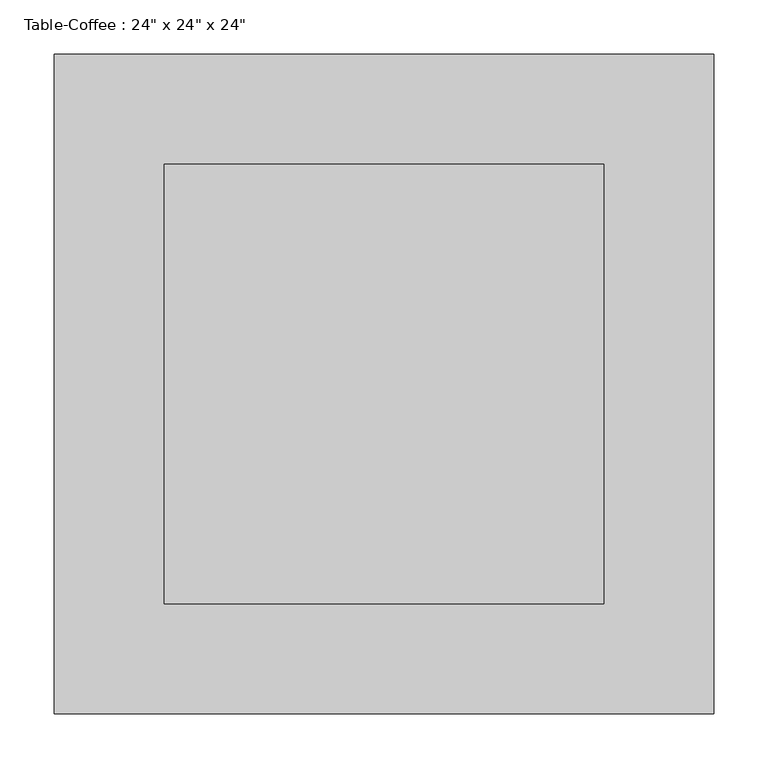
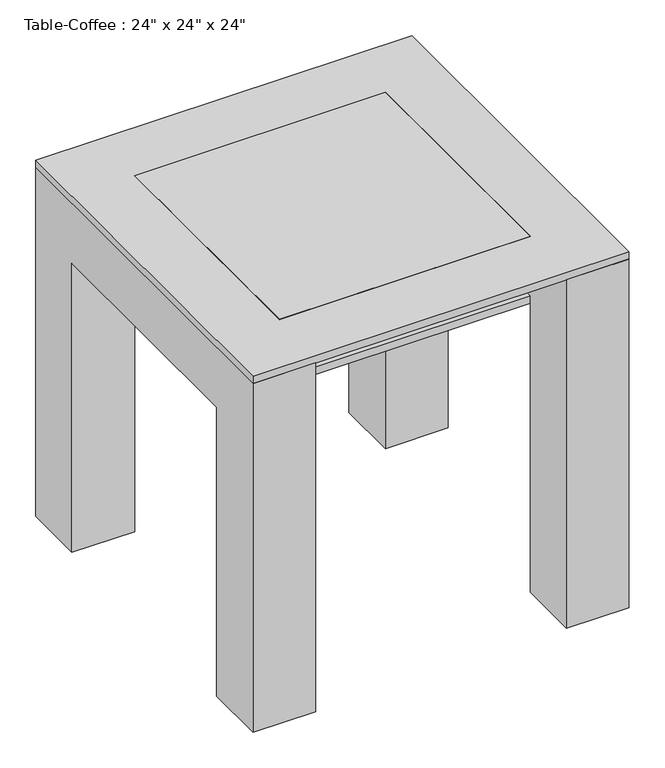
"""IFC4 building model written with IfcOpenShell, lengths in millimetres: furniture geometry."""

from ifc_helpers import new_model, si_unit, frame, origin, place, context, project, spatial, polyline, outline, extrude, source, transform, mapped, element, save


def furniture_b5c51a22(model_context):
    return source(origin(), model_context, "Body", "SweptSolid", [
        extrude(outline(polyline([(221.4657667, 298.4110778), (221.4657667, -107.9889222), (-184.9342333, -107.9889222), (-184.9342333, 298.4110778), (221.4657667, 298.4110778)])), frame((0.0, 0.0, 495.3), z_axis=(0.0, 0.0, 1.0), x_axis=(1.0, 0.0, 0.0)), (0.0, 0.0, 1.0), 12.7),
        extrude(outline(polyline([(400.0110778, 0.0), (298.4110778, 0.0), (298.4110778, 495.3), (-107.9889222, 495.3), (-107.9889222, 0.0), (-209.5889222, 0.0), (-209.5889222, 596.9), (400.0110778, 596.9), (400.0110778, 0.0)])), frame((221.4657667, 0.0, 0.0), z_axis=(1.0, 0.0, 0.0), x_axis=(0.0, 1.0, 0.0)), (0.0, 0.0, 1.0), 101.6),
        extrude(outline(polyline([(400.0110778, 596.9), (400.0110778, 0.0), (298.4110778, 0.0), (298.4110778, 495.3), (-107.9889222, 495.3), (-107.9889222, 0.0), (-209.5889222, 0.0), (-209.5889222, 596.9), (400.0110778, 596.9)])), frame((-286.5342333, 0.0, 0.0), z_axis=(1.0, 0.0, 0.0), x_axis=(0.0, 1.0, 0.0)), (0.0, 0.0, 1.0), 101.6),
        extrude(outline(polyline([(221.4657667, 298.4110778), (221.4657667, -107.9889222), (-184.9342333, -107.9889222), (-184.9342333, 298.4110778), (221.4657667, 298.4110778)])), frame((0.0, 0.0, 596.9), z_axis=(0.0, 0.0, 1.0), x_axis=(1.0, 0.0, 0.0)), (0.0, 0.0, 1.0), 12.7),
        extrude(outline(polyline([(323.0657667, 400.0110778), (323.0657667, -209.5889222), (-286.5342333, -209.5889222), (-286.5342333, 400.0110778), (323.0657667, 400.0110778)]), holes=[polyline([(221.4657667, 298.4110778), (-184.9342333, 298.4110778), (-184.9342333, -107.9889222), (221.4657667, -107.9889222), (221.4657667, 298.4110778)])]), frame((0.0, 0.0, 596.9), z_axis=(0.0, 0.0, 1.0), x_axis=(1.0, 0.0, 0.0)), (0.0, 0.0, 1.0), 12.7),
    ])


if __name__ == "__main__":
    model = new_model("IFC4")
    model_context = context("Model", 3, world=origin())
    ifc_project = project(units=[si_unit("LENGTHUNIT", "METRE", prefix="MILLI")], contexts=[model_context])
    site = spatial("IfcSite", under=ifc_project)
    building = spatial("IfcBuilding", under=site)
    placement = place(None, origin())
    furniture_shape = furniture_b5c51a22(model_context)
    element("IfcFurniture", 1, ObjectType="Table-Coffee : 24\" x 24\" x 24\"", at=placement, inside=building, context=model_context, shape_type="MappedRepresentation", body=[
        mapped(furniture_shape, transform((0.0, 0.0, 0.0), x_axis=(1.0, 0.0, 0.0), y_axis=(0.0, 1.0, 0.0), z_axis=(0.0, 0.0, 1.0))),
    ])
    save(model, "model.ifc")

# Revit data of these elements
# Type "Table-Coffee : 24\" x 24\" x 24\""
#   Assembly Code = "E2020200"
#   Height = 2' - 0"
#   Length = 2' - 0"
#   Width = 2' - 0"
#   Top Material = none
#   Frame Material = none
# Element 1 (IfcFurniture, "Table-Coffee : 24\" x 24\" x 24\"")
#   Materials on its faces: "Glass - Clear, Grey"
# Materials
#   "Glass - Clear, Grey": class "Glass", colour RGB 252 255 255, transparency 0.64
